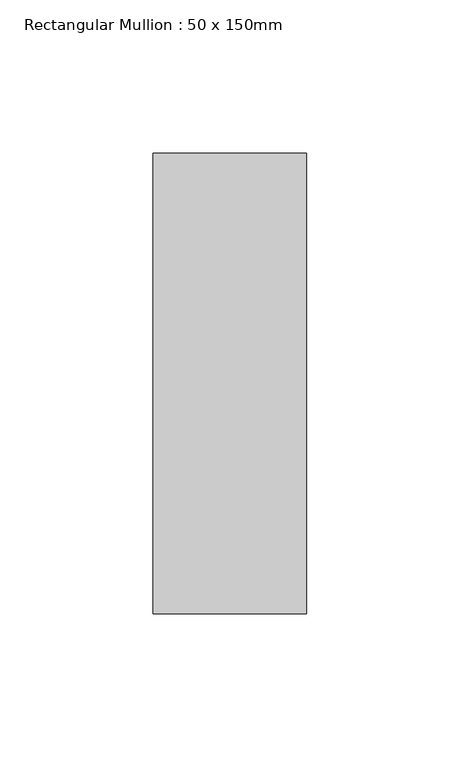
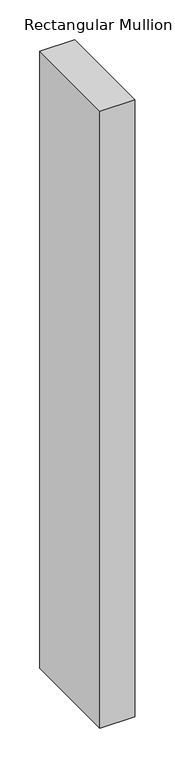
"""IFC4 building model written with IfcOpenShell, lengths in millimetres: member geometry, Rectangular Mullion : 50 x 150mm."""

from ifc_helpers import new_model, si_unit, frame, origin, place, context, project, spatial, polyline, outline, extrude, source, transform, mapped, element, save


def rectangular_mullion_50_x_150mm_a5bab1e1(model_context):
    return source(origin(), model_context, "Body", "SweptSolid", [
        extrude(outline(polyline([(25.0, 75.0), (25.0, -75.0), (-25.0, -75.0), (-25.0, 75.0), (25.0, 75.0)])), frame((0.0, 0.0, -941.6666667), z_axis=(0.0, 0.0, 1.0), x_axis=(1.0, 0.0, 0.0)), (0.0, 0.0, 1.0), 941.6666667),
    ])


if __name__ == "__main__":
    model = new_model("IFC4")
    model_context = context("Model", 3, world=origin())
    ifc_project = project(units=[si_unit("LENGTHUNIT", "METRE", prefix="MILLI")], contexts=[model_context])
    site = spatial("IfcSite", under=ifc_project)
    building = spatial("IfcBuilding", under=site)
    placement = place(None, origin())
    rectangular_mullion_50_x_150mm_shape = rectangular_mullion_50_x_150mm_a5bab1e1(model_context)
    element("IfcMember", 1, ObjectType="Rectangular Mullion : 50 x 150mm", at=placement, inside=building, context=model_context, shape_type="MappedRepresentation", body=[
        mapped(rectangular_mullion_50_x_150mm_shape, transform((0.0, 0.0, 0.0), x_axis=(1.0, 0.0, 0.0), y_axis=(0.0, 1.0, 0.0), z_axis=(0.0, 0.0, 1.0))),
    ])
    save(model, "model.ifc")

# Revit data of these elements
# Type "Rectangular Mullion : 50 x 150mm"
#   built-in parameter 1007304 = 0.492126 (stored number, unit not read)
#   built-in parameter 1007301 = 0.082021 (stored number, unit not read)
#   built-in parameter 1007300 = 0.082021 (stored number, unit not read)
# Element 1 (IfcMember, "Rectangular Mullion : 50 x 150mm")
#   Materials on its faces: "Aluminium"
# Materials
#   "Aluminium": class "Metal", colour RGB 247 247 247, transparency 0, Description = "Aluminium 6061", Cost = 0
